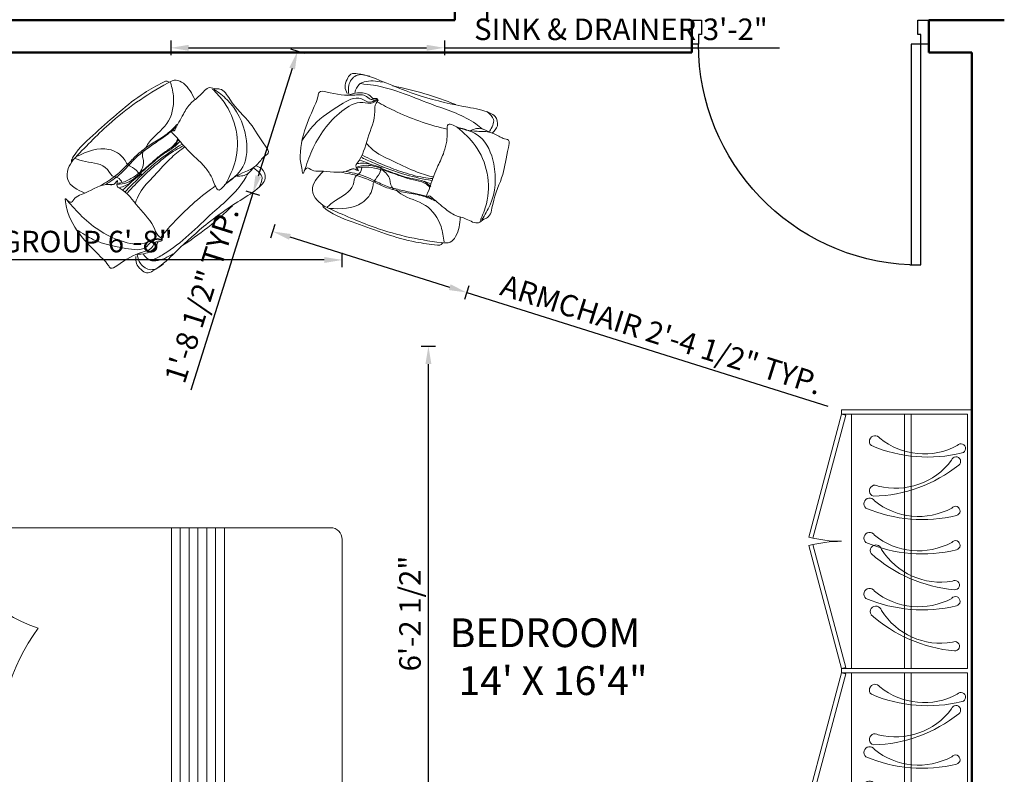
# Model space of a CAD drawing. Units: inches. Extents: x 1961 to 3038, y 800 to 1438.
# Tile 3 of 13: x 2666 to 2803, y 953 to 1058. Entities that reach past the tile are written whole.
import ezdxf

# ---------------------------------------------------------------- set-up
doc = ezdxf.new("R2010")
doc.units = ezdxf.units.IN
for name, color, linetype, lineweight in [('A-ANNO-DIMS', 2, 'Continuous', 18), ('A-AREA-IDEN', 7, 'Continuous', 25), ('A-DOOR', 3, 'Continuous', 25), ('A-FURN', 8, 'Continuous', 18), ('A-WALL', 7, 'Continuous', 50)]:
    doc.layers.add(name, color=color, linetype=linetype, lineweight=lineweight)
doc.styles.get("Standard").update_dxf_attribs({"font": 'arial.ttf'})
doc.dimstyles.new('ISO-25', dxfattribs={"dimtxt": 3, "dimasz": 2.5, "dimexe": 1, "dimexo": 1, "dimtad": 1, "dimdec": 4, "dimlunit": 4, "dimtxsty": 'Standard', "dimcen": 2.5, "dimadec": 0, "dimazin": 0, "dimtfac": 1, "dimtdec": 4, "dimtmove": 0, "dimatfit": 3, "dimfxl": 1, "dimfxlon": 1, "dimarcsym": 0})

# ---------------------------------------------------------------- blocks, each defined once
blk = doc.blocks.new('A$C41DA168A')
for p, q in [((151.4, 2380), (0, 1814.9)), ((19.3, 1809.8), (170.7, 2374.8)), ((151.4, 2380), (151.4, 2400)), ((151.4, 2400), (751.4, 2400)), ((731.4, 2380), (151.4, 2380)), ((170.7, 2374.8), (151.4, 2380)), ((196.6, 1210), (196.6, 2380)), ((441.4, 1210), (441.4, 2380)), ((471.4, 1210), (471.4, 2380)), ((731.4, 1210), (731.4, 2380)), ((751.4, 2400), (751.4, 0)), ((0, 1814.9), (19.3, 1809.8)), ((0, 1775.1), (19.3, 1780.2)), ((151.4, 1210), (0, 1775.1)), ((19.3, 1780.2), (170.7, 1215.2)), ((151.4, 1190), (0, 624.9)), ((19.3, 619.8), (170.7, 1184.8)), ((170.7, 1215.2), (151.4, 1210)), ((151.4, 1210), (731.4, 1210)), ((151.4, 1190), (151.4, 1210)), ((731.4, 1190), (151.4, 1190)), ((170.7, 1184.8), (151.4, 1190)), ((196.6, 20), (196.6, 1190)), ((441.4, 1190), (441.4, 20)), ((471.4, 1190), (471.4, 20)), ((731.4, 20), (731.4, 1190)), ((0, 624.9), (19.3, 619.8)), ((0, 585.1), (19.3, 590.2)), ((19.3, 590.2), (170.7, 25.2)), ((151.4, 20), (0, 585.1)), ((170.7, 25.2), (151.4, 20)), ((151.4, 0), (151.4, 20)), ((151.4, 20), (731.4, 20)), ((751.4, 0), (151.4, 0))]:
    blk.add_line(p, q)
for centre, radius, start, end in [((305.7, 2255.1), 26.3, 32.2752, 228.9651), ((530.9, 2518.7), 321.7, 230.8748, 298.3986), ((548.2, 2849.7), 667, 247.0836, 283.6394), ((700.5, 2222.3), 21.4, 283.2942, 141.1703), ((677.9, 2162.6), 21.4, 307.9992, 165.8752), ((277.3, 2668.9), 667, 271.7885, 308.3443), ((399.9, 2361), 321.7, 255.5797, 323.1036), ((305.5, 2027.4), 26.3, 56.9801, 253.67), ((280.2, 1967.6), 26.3, 32.2752, 228.9651), ((505.3, 2231.2), 321.7, 230.8748, 298.3986), ((675, 1934.8), 21.4, 283.2942, 141.1703), ((522.6, 2562.2), 667, 247.0836, 283.6394), ((151.4, 2380), 585, 255, 270), ((280.2, 1809.7), 26.3, 32.2752, 228.9651), ((505.3, 2073.2), 321.7, 230.8748, 298.3986), ((151.4, 1210), 585, 90, 105), ((522.6, 2404.2), 667, 247.0836, 283.6394), ((309.6, 1752), 26.3, 13.455, 210.1449), ((675, 1776.9), 21.4, 283.2942, 141.1703), ((730.9, 2236.5), 667, 228.2634, 264.8192), ((607.8, 1928.8), 321.7, 212.0546, 279.5785), ((672.7, 1593.6), 21.4, 264.474, 122.3501), ((280.2, 1552.2), 26.3, 32.2752, 228.9651), ((505.3, 1815.7), 321.7, 230.8748, 298.3986), ((675, 1519.4), 21.4, 283.2942, 141.1703), ((522.6, 2146.7), 667, 247.0836, 283.6394), ((309.6, 1470.8), 26.3, 13.455, 210.1449), ((730.9, 1955.3), 667, 228.2634, 264.8192), ((607.8, 1647.6), 321.7, 212.0546, 279.5785), ((672.7, 1312.3), 21.4, 264.474, 122.3501), ((305.7, 1111), 26.3, 32.2752, 228.9651), ((548.2, 1705.5), 667, 247.0836, 283.6394), ((530.9, 1374.6), 321.7, 230.8748, 298.3986), ((700.5, 1078.2), 21.4, 283.2942, 141.1703), ((277.3, 1524.8), 667, 271.7885, 308.3443), ((399.9, 1216.9), 321.7, 255.5797, 323.1036), ((677.9, 1018.5), 21.4, 307.9992, 165.8752), ((305.5, 883.3), 26.3, 56.9801, 253.67), ((280.2, 823.5), 26.3, 32.2752, 228.9651), ((505.3, 1087.1), 321.7, 230.8748, 298.3986), ((522.6, 1418), 667, 247.0836, 283.6394), ((675, 790.7), 21.4, 283.2942, 141.1703), ((280.2, 665.6), 26.3, 32.2752, 228.9651), ((505.3, 929.1), 321.7, 230.8748, 298.3986), ((522.6, 1260.1), 667, 247.0836, 283.6394), ((675, 632.8), 21.4, 283.2942, 141.1703), ((309.6, 607.9), 26.3, 13.455, 210.1449), ((730.9, 1092.4), 667, 228.2634, 264.8192), ((607.8, 784.7), 321.7, 212.0546, 279.5785), ((672.7, 449.5), 21.4, 264.474, 122.3501), ((280.2, 408.1), 26.3, 32.2752, 228.9651), ((505.3, 671.6), 321.7, 230.8748, 298.3986), ((522.6, 1002.6), 667, 247.0836, 283.6394), ((675, 375.3), 21.4, 283.2942, 141.1703), ((309.6, 326.7), 26.3, 13.455, 210.1449), ((607.8, 503.5), 321.7, 212.0546, 279.5785), ((730.9, 811.2), 667, 228.2634, 264.8192), ((672.7, 168.2), 21.4, 264.474, 122.3501)]:
    blk.add_arc(centre, radius, start, end)
blk = doc.blocks.new('A$C11850ECD')
for p, q in [((0, 1.95), (0, 0.04)), ((0, 1.95), (1.2, 1.95)), ((1.2, 1.95), (1.2, 0.04)), ((1.2318, 1.952), (1.8168, 1.952)), ((1.2318, 1.367), (1.2318, 1.952)), ((1.5243, 1.952), (1.5243, 1.7225)), ((1.8168, 1.952), (1.8168, 1.367)), ((0, 1.91), (1.2, 1.91)), ((0, 1.9), (1.2, 1.9)), ((1.4613, 1.6586), (1.2318, 1.6586)), ((1.8168, 1.6595), (1.5873, 1.6595)), ((1.5243, 1.5965), (1.5243, 1.367)), ((1.8168, 1.367), (1.2318, 1.367)), ((0, 0.58), (1.2, 0.58)), ((0, 0.55), (1.2, 0.55)), ((0, 0.52), (1.2, 0.52)), ((0, 0.49), (1.2, 0.49)), ((0, 0.46), (1.2, 0.46)), ((0, 0.43), (1.2, 0.43)), ((0, 0.4), (1.2, 0.4)), ((1.16, 0), (0.04, 0))]:
    blk.add_line(p, q)
for radius in [0.27, 0.09]:
    blk.add_circle((1.5243, 1.6595), radius)
for centre, radius, start, end in [((-0.2053, 1.694), 0.5605, 346.15, 13.85), ((0.5998, 5.1077), 3.2899, 265.4501, 274.5499), ((0.3425, 1.5416), 0.3789, 4.7708, 46.8165), ((0.3425, 1.5416), 0.4089, 4.1373, 42.5614), ((0.3425, 1.5416), 0.4389, 3.5318, 39.1874), ((0.3425, 1.5416), 0.4689, 2.9489, 36.4321), ((1.3429, 1.694), 0.5004, 164.4468, 195.5532), ((0.5998, -0.4629), 2.0395, 82.6483, 97.3517), ((0.8389, 0.3894), 1.0202, 69.2731, 145.3133), ((1.3044, 0.8859), 0.4695, 102.8515, 161.769), ((0.4655, 0.5058), 0.6574, 53.2823, 135.0802), ((0.04, 0.04), 0.04, 180, 270), ((1.16, 0.04), 0.04, 270, 0)]:
    blk.add_arc(centre, radius, start, end)
blk = doc.blocks.new('A$C4F7F6E58')
at = {"ltscale": 0.8}
blk.add_arc((588.7, 1807.5), 1799.5, 263.3519, 274.6778, dxfattribs=at)
for points, knots in [([(212.3, 745.6), (213, 747.1), (218.5, 755.7), (289.3, 782.2), (464.8, 786.6), (683, 801.1), (833.5, 773.4), (885.9, 762.1), (890.8, 751.2), (892, 745.8)], [17.99656, 17.99656, 17.99656, 17.99656, 24.654541, 59.355785, 289.542515, 728.551681, 882.30278, 904.288941, 924.788376, 924.788376, 924.788376, 924.788376]), ([(227.7, 750.3), (210.2, 745.1), (173.8, 734.3), (112.7, 672.2), (142.7, 611.7), (162.7, 571.5)], [0, 0, 0, 0, 71.10826, 148.314414, 301.164142, 301.164142, 301.164142, 301.164142]), ([(227.7, 750.3), (317.7, 761.3), (538, 788.2), (765.4, 771.9), (932.7, 737.6), (960.4, 670.7), (949, 620.8), (940.8, 585)], [0, 0, 0, 0, 350.70006, 858.205579, 917.075962, 972.848208, 1113.682742, 1113.682742, 1113.682742, 1113.682742]), ([(238.5, 752.4), (248.9, 735.1), (280.7, 682.5), (353.2, 623), (328.1, 546.3), (358.7, 520.1), (356, 500.2), (354.3, 487.1)], [0, 0, 0, 0, 79.489254, 242.739997, 314.65082, 339.438853, 386.590051, 386.590051, 386.590051, 386.590051]), ([(251.9, 753.3), (314, 736.9), (407.7, 709), (450.5, 599.8), (436.6, 550.7), (446.8, 516.8), (458.3, 488.6), (454.8, 465.3), (454.1, 460.2)], [14.22546, 14.22546, 14.22546, 14.22546, 248.732969, 375.734785, 418.155281, 441.003934, 511.971111, 531.951261, 531.951261, 531.951261, 531.951261]), ([(897.7, 739.5), (885.8, 714.1), (853.7, 645.7), (745.6, 561.4), (631.8, 577.3), (575.9, 554.3), (565.2, 549.9)], [0, 0, 0, 0, 109.257629, 294.294606, 484.078985, 528.781997, 528.781997, 528.781997, 528.781997]), ([(85.7, 579.8), (108.8, 591.2), (183.8, 558.4), (269.7, 555.1), (310.5, 503.2), (358.6, 519.6), (314.2, 495.4), (342.8, 432.7), (331.4, 330.5), (346.7, 210.6), (316.5, 146.3), (334, 110.2), (306.1, 110.8), (292.3, 132.5), (251.9, 105.6), (169.8, 145.3), (100.6, 155.5), (8.5, 162.1), (15.1, 200), (9.7, 271), (-8.6, 395.1), (11.8, 535.4), (46.6, 590.2), (64.4, 626.1), (63, 591.9), (73.2, 578.8), (82.8, 578.4), (85.7, 579.8)], [0, 0, 0, 0, 100.597406, 281.319891, 315.054718, 349.509689, 389.200281, 408.162693, 598.959573, 792.637569, 852.601939, 880.830983, 902.666946, 929.495226, 968.022274, 1050.611483, 1254.96923, 1301.260424, 1329.316584, 1382.311494, 1591.546287, 1820.820862, 1871.094845, 1893.578982, 1925.370652, 1945.336599, 1957.814292, 1957.814292, 1957.814292, 1957.814292]), ([(64.1, 601.9), (65, 562.5), (67.9, 434.1), (120.6, 270.6), (224.7, 149.7), (303.4, 150.5), (317.5, 124.2), (323, 114)], [0, 0, 0, 0, 153.199383, 498.931474, 658.942203, 726.134726, 768.614124, 768.614124, 768.614124, 768.614124]), ([(752, 526.5), (782.1, 539.3), (834.3, 561.4), (909.8, 589.7), (975.3, 580.2), (1040.8, 601.3), (1061.5, 560.1), (1098.2, 533.5), (1075.6, 429.8), (1100.1, 301), (1076.9, 198.1), (1073.4, 103.2), (1039.5, 112.8), (1006.2, 107.3), (957.4, 94.2), (871.3, 124.9), (803.4, 133.9), (712.9, 116.6), (740.5, 179.9), (750.1, 225.2), (754, 285.2), (740.4, 365.6), (734.8, 446.5), (737.4, 494.3), (727.2, 554.4), (746.7, 524.2), (752, 526.5)], [0, 0, 0, 0, 127.427681, 224.276404, 302.261986, 392.779016, 437.096694, 463.557063, 563.507143, 784.838909, 976.246821, 1028.506194, 1069.058754, 1082.809516, 1162.638681, 1258.731906, 1422.314775, 1462.867277, 1544.873185, 1583.434163, 1661.617215, 1768.019408, 1911.553131, 1945.84397, 1998.930645, 2021.420543, 2021.420543, 2021.420543, 2021.420543]), ([(253, 547.9), (286.3, 543.8), (348.1, 536.3), (432.8, 543.6), (496.9, 552.8), (560.5, 553.7), (630.5, 546.9), (709.3, 534), (761.1, 540.1), (783.5, 542.8)], [0, 0, 0, 0, 130.481225, 241.871234, 329.653071, 382.635961, 489.129551, 603.809277, 691.391283, 691.391283, 691.391283, 691.391283]), ([(279.6, 536), (309.9, 532.6), (359.7, 527), (435.7, 535.5), (505.5, 548.5), (584.2, 543.4), (656.3, 537.7), (718.8, 532.6), (754.3, 534.8), (769.2, 535.7)], [0, 0, 0, 0, 118.476382, 194.076844, 297.117853, 393.933927, 499.659542, 579.515716, 637.850776, 637.850776, 637.850776, 637.850776]), ([(551.9, 549.7), (549.4, 547.7), (542.3, 542.2), (527, 531), (516.3, 490.8), (483.3, 477.5), (459.7, 467.9)], [0, 0, 0, 0, 12.396318, 35.253043, 71.848794, 163.317226, 163.317226, 163.317226, 163.317226]), ([(1056.3, 563.2), (1063.7, 533.8), (1089.5, 431.8), (1051.6, 268.9), (926.4, 121.9), (821.2, 125.9), (773.1, 127.7)], [0, 0, 0, 0, 117.484834, 407.414781, 620.246611, 799.395046, 799.395046, 799.395046, 799.395046]), ([(1050, 569.3), (1052.8, 537.7), (1065, 399.7), (962.6, 208.3), (822.2, 146.8), (780.2, 128.4)], [0, 0, 0, 0, 123.587716, 539.784626, 717.53011, 717.53011, 717.53011, 717.53011]), ([(325.5, 498.4), (341, 486.6), (382.1, 460.9), (458.6, 463.7), (543.1, 467.4), (620.7, 469.4), (690.3, 455.1), (724.9, 469.5), (738.9, 475.3)], [49.606189, 49.606189, 49.606189, 49.606189, 124.052713, 239.571345, 333.3214, 456.942517, 542.38691, 600.329448, 600.329448, 600.329448, 600.329448]), ([(328.4, 501.8), (338.5, 496), (366.7, 480), (433, 469.7), (510.6, 467.3), (589.8, 472.9), (650.9, 468.8), (701.4, 464), (726.3, 476.5), (736.2, 481.5)], [0, 0, 0, 0, 45.174964, 125.558829, 256.610972, 349.076861, 433.189907, 497.197145, 539.983253, 539.983253, 539.983253, 539.983253]), ([(2.6, 449.8), (13.4, 414.5), (41.8, 321.3), (126.7, 222.3), (214.2, 117.7), (295.4, 153.1), (311.3, 117.2), (325.2, 118), (331.2, 118.3)], [0, 0, 0, 0, 141.86292, 373.630524, 526.427539, 601.735045, 630.296438, 651.966247, 651.966247, 651.966247, 651.966247]), ([(323.9, 476.4), (335.1, 471.9), (362.5, 460.9), (411, 458.3), (446.9, 458.3), (465.4, 458.3)], [0, 0, 0, 0, 46.593931, 114.59593, 186.8347, 186.8347, 186.8347, 186.8347]), ([(330.8, 455.3), (347.2, 455.7), (369, 456.2), (390.6, 458.7), (395.9, 459.3)], [0, 0, 0, 0, 63.690529, 84.680578, 84.680578, 84.680578, 84.680578]), ([(338.1, 439.1), (365.6, 442.5), (450.6, 453.1), (583.9, 460.6), (688.5, 449), (735.4, 443.9)], [0, 0, 0, 0, 108.049196, 333.891802, 517.629591, 517.629591, 517.629591, 517.629591]), ([(339.5, 358.4), (356.3, 367.8), (409.4, 397.6), (517.2, 404.8), (632.4, 427.1), (708.8, 424.4), (739.9, 423.2)], [0, 0, 0, 0, 74.526832, 235.368216, 411.08678, 532.069418, 532.069418, 532.069418, 532.069418]), ([(340.4, 426.7), (378.9, 432.1), (452.3, 442.3), (568.3, 448.5), (663.3, 447.1), (721.2, 435), (737.7, 431.5)], [0, 0, 0, 0, 151.37946, 288.564606, 452.874576, 518.766039, 518.766039, 518.766039, 518.766039]), ([(326.5, 126.4), (359.8, 134.8), (489.4, 155.9), (624.9, 163.3), (724.8, 154.9), (728.6, 154.6)], [89.052228, 89.052228, 89.052228, 89.052228, 222.96578, 599.021538, 613.61065, 613.61065, 613.61065, 613.61065]), ([(158.9, 133), (150.2, 123.2), (131.9, 102.7), (133.9, 63.3), (141.9, 22.3), (217.8, 4.9), (345.6, 16.6), (555.4, 32.4), (757.1, 15.8), (894.9, -4.6), (965.2, 8.9), (992.9, 55.8), (976.8, 87.4), (969, 102.7)], [0, 0, 0, 0, 48.943013, 103.025949, 148.534553, 195.328972, 375.361256, 667.155028, 1003.182997, 1165.538814, 1206.58239, 1274.47318, 1338.225006, 1338.225006, 1338.225006, 1338.225006]), ([(169.5, 134.2), (162.3, 119.5), (145.6, 84.9), (169.5, 11.7), (220.8, 8.8), (248.3, 7.3)], [0, 0, 0, 0, 62.883797, 147.829924, 245.663948, 245.663948, 245.663948, 245.663948]), ([(165.8, 141.2), (180, 130.6), (212.9, 106.1), (268, 97.7), (294.2, 114.6), (300.7, 118.8)], [0, 0, 0, 0, 69.56601, 160.233414, 189.860891, 189.860891, 189.860891, 189.860891]), ([(196.7, 116), (197, 98.2), (197.4, 70), (245.3, 28.7), (288.9, 22), (322.6, 16.8)], [0, 0, 0, 0, 65.355661, 103.354857, 233.394712, 233.394712, 233.394712, 233.394712]), ([(855.5, 122.2), (863.4, 115.5), (886.8, 95.7), (925.1, 92.8), (947, 101), (950.1, 102.2)], [0, 0, 0, 0, 40.128951, 118.809172, 131.501248, 131.501248, 131.501248, 131.501248]), ([(912.5, 96.7), (898.4, 91.1), (808.6, 55.2), (592.1, 57.5), (371.7, 28.4), (235.4, 55.8), (212.6, 60.4)], [0, 0, 0, 0, 58.661068, 375.93507, 825.814021, 916.361162, 916.361162, 916.361162, 916.361162]), ([(952.5, 98), (958.3, 72.4), (968.9, 25.7), (925.9, 8), (906.6, 0)], [0, 0, 0, 0, 88.639768, 160.999132, 160.999132, 160.999132, 160.999132])]:
    blk.add_open_spline(points, degree=3, knots=knots, dxfattribs=at)
for points in [[(295.1, 523.4), (300.3, 519), (305.5, 514.5), (310.7, 510.2)], [(736.1, 462.3), (723.2, 461.1), (710.3, 459.9), (697.4, 458.7)]]:
    blk.add_open_spline(points, degree=3, dxfattribs=at)
blk = doc.blocks.new('DOOR-SWING-33IN')
for p, q in [((30.36, 34.07), (31.87, 34.07)), ((30.53, 3.34), (30.53, 34.07)), ((31.87, 34.07), (31.87, 3.34)), ((33, 3.34), (30.53, 3.34)), ((31.87, 3.34), (31.87, 2)), ((31.87, 2), (31.46, 2)), ((31.46, 2), (31.46, 0)), ((31.46, 0), (33, 0))]:
    blk.add_line(p, q)
blk.add_lwpolyline([(0, 0), (1.34, 0), (1.34, 2), (0.93, 2), (0.93, 3.34), (0, 3.34)])
blk.add_arc((31.69, 3.34), 30.76, 92.4896, 180)
blk = doc.blocks.new('*D39')
at = {"layer": 'A-ANNO-DIMS', "color": 0, "lineweight": -2, "transparency": 16777216}
for p, q in [((2701.72, 1029.95), (2701.12, 1028.04)), ((2703.81, 1028.24), (2726.04, 1021.24)), ((2728.73, 1021.44), (2728.13, 1019.53)), ((2728.43, 1020.49), (2778.71, 1004.65))]:
    blk.add_line(p, q, dxfattribs=at)
at = {"layer": 'A-ANNO-DIMS', "color": 0, "transparency": 16777216}
for points in [[(2703.93, 1028.64), (2703.68, 1027.85), (2701.42, 1028.99)], [(2726.17, 1021.64), (2725.92, 1020.84), (2728.43, 1020.49)]]:
    blk.add_solid(points, dxfattribs=at)
at = {"layer": 'Defpoints', "color": 0, "transparency": 16777216}
for p in [(2702.7, 1033.05), (2729.7, 1024.54), (2728.43, 1020.49)]:
    blk.add_point(p, dxfattribs=at)
at = {"layer": 'A-ANNO-DIMS', "color": 0, "transparency": 16777216, "insert": (2755.42, 1014.27), "char_height": 3, "attachment_point": 5, "rotation": 342.5185}
blk.add_mtext('ARMCHAIR 2\'-4 1/2" TYP.', dxfattribs=at)
blk = doc.blocks.new('*D40')
at = {"layer": 'A-ANNO-DIMS', "color": 0, "lineweight": -2, "transparency": 16777216}
for p, q in [((2705.82, 1053.76), (2703.91, 1054.36)), ((2704.11, 1051.68), (2699.4, 1036.71)), ((2698.65, 1034.32), (2690.01, 1006.9)), ((2699.6, 1034.02), (2697.69, 1034.62))]:
    blk.add_line(p, q, dxfattribs=at)
at = {"layer": 'A-ANNO-DIMS', "color": 0, "transparency": 16777216}
for points in [[(2703.71, 1051.8), (2704.51, 1051.55), (2704.86, 1054.06)], [(2699, 1036.83), (2699.79, 1036.58), (2698.65, 1034.32)]]:
    blk.add_solid(points, dxfattribs=at)
at = {"layer": 'Defpoints', "color": 0, "transparency": 16777216}
for p in [(2708.91, 1052.78), (2698.65, 1034.32), (2702.7, 1033.05)]:
    blk.add_point(p, dxfattribs=at)
at = {"layer": 'A-ANNO-DIMS', "color": 0, "transparency": 16777216, "insert": (2691.88, 1020.07), "char_height": 3, "attachment_point": 5, "rotation": 72.5185}
blk.add_mtext('1\'-8 1/2" TYP.', dxfattribs=at)
blk = doc.blocks.new('*D57')
at = {"layer": 'A-ANNO-DIMS', "color": 0, "lineweight": -2, "transparency": 16777216}
for p, q in [((2631.09, 1024.03), (2631.09, 1026.03)), ((2711.09, 1024.03), (2711.09, 1026.03)), ((2708.59, 1025.03), (2633.59, 1025.03))]:
    blk.add_line(p, q, dxfattribs=at)
at = {"layer": 'A-ANNO-DIMS', "color": 0, "transparency": 16777216}
for points in [[(2633.59, 1025.44), (2633.59, 1024.61), (2631.09, 1025.03)], [(2708.59, 1025.44), (2708.59, 1024.61), (2711.09, 1025.03)]]:
    blk.add_solid(points, dxfattribs=at)
at = {"layer": 'Defpoints', "color": 0, "transparency": 16777216}
for p in [(2631.09, 1025.03), (2631.09, 1013.03), (2711.09, 1013.03)]:
    blk.add_point(p, dxfattribs=at)
at = {"layer": 'A-ANNO-DIMS', "color": 0, "transparency": 16777216, "insert": (2671.09, 1027.2), "char_height": 3, "attachment_point": 5}
blk.add_mtext('BED GROUP 6\'-8"', dxfattribs=at)
blk = doc.blocks.new('*D58')
at = {"layer": 'A-ANNO-DIMS', "color": 0, "lineweight": -2, "transparency": 16777216}
for p, q in [((2722.09, 1013.03), (2724.09, 1013.03)), ((2723.09, 941.07), (2723.09, 1010.53)), ((2722.09, 938.57), (2724.09, 938.57))]:
    blk.add_line(p, q, dxfattribs=at)
at = {"layer": 'A-ANNO-DIMS', "color": 0, "transparency": 16777216}
for points in [[(2722.67, 1010.53), (2723.5, 1010.53), (2723.09, 1013.03)], [(2722.67, 941.07), (2723.5, 941.07), (2723.09, 938.57)]]:
    blk.add_solid(points, dxfattribs=at)
at = {"layer": 'Defpoints', "color": 0, "transparency": 16777216}
for p in [(2711.09, 1013.03), (2723.09, 1013.03), (2711.09, 938.57)]:
    blk.add_point(p, dxfattribs=at)
at = {"layer": 'A-ANNO-DIMS', "color": 0, "transparency": 16777216, "insert": (2720.91, 975.8), "char_height": 3, "attachment_point": 5, "rotation": 90}
blk.add_mtext('6\'-2 1/2"', dxfattribs=at)
blk = doc.blocks.new('*D69')
at = {"layer": 'A-ANNO-DIMS', "color": 0, "lineweight": -2, "transparency": 16777216}
for p, q in [((2687.2, 1055.56), (2687.2, 1053.56)), ((2689.7, 1054.56), (2722.82, 1054.56)), ((2725.32, 1055.56), (2725.32, 1053.56)), ((2725.32, 1054.56), (2771.96, 1054.56))]:
    blk.add_line(p, q, dxfattribs=at)
at = {"layer": 'A-ANNO-DIMS', "color": 0, "transparency": 16777216}
for points in [[(2689.7, 1054.98), (2689.7, 1054.15), (2687.2, 1054.56)], [(2722.82, 1054.98), (2722.82, 1054.15), (2725.32, 1054.56)]]:
    blk.add_solid(points, dxfattribs=at)
at = {"layer": 'Defpoints', "color": 0, "transparency": 16777216}
for p in [(2687.2, 1060.28), (2725.32, 1060.28), (2725.32, 1054.56)]:
    blk.add_point(p, dxfattribs=at)
at = {"layer": 'A-ANNO-DIMS', "color": 0, "transparency": 16777216, "insert": (2749.89, 1056.75), "char_height": 3, "attachment_point": 5}
blk.add_mtext('SINK & DRAINER 3\'-2"', dxfattribs=at)

msp = doc.modelspace()

# ---------------------------------------------------------------- linework, layer by layer
at = {"layer": 'A-WALL'}
for p, q in [((2726.76803, 1124.41975), (2726.76803, 1058.41975)), ((2731.26803, 1124.41975), (2731.26803, 1058.41975)), ((2726.76803, 1058.41975), (2630.76803, 1058.41975)), ((2759.76803, 1058.41975), (2759.76803, 1053.91975)), ((2803.26803, 1058.41975), (2792.76803, 1058.41975)), ((2792.76803, 1058.41975), (2792.76803, 1053.91975)), ((2759.76803, 1053.91975), (2630.76803, 1053.91975)), ((2798.76803, 1053.91975), (2792.76803, 1053.91975)), ((2798.76803, 1053.91975), (2798.76803, 858.91975))]:
    msp.add_line(p, q, dxfattribs=at)

# ---------------------------------------------------------------- block references
at = {"layer": 'A-DOOR', "extrusion": (0, 0, -1), "zscale": -1, "rotation": 180}
msp.add_blockref('DOOR-SWING-33IN', (-2759.768, 1058.41951), dxfattribs=at)
at = {"layer": 'A-FURN'}
for name, p, xscale, yscale, zscale, rotation in [('A$C4F7F6E58', (2681.36471, 1020.26477), 0.0258216611436376, 0.0258216611436376, 0.0258216611436376, 39.33090782219615), ('A$C4F7F6E58', (2708.89155, 1052.70849), -0.0258216611436376, 0.0258216611436376, 0.0258216611436376, 162.5185450702014), ('A$C11850ECD', (2711.08548, 938.57032), 40.98381615062051, 40.98381615062051, 40.98381615062051, 90)]:
    msp.add_blockref(name, p, dxfattribs=dict(at, xscale=xscale, yscale=yscale, zscale=zscale, rotation=rotation))
at = {"layer": 'A-FURN', "xscale": 0.0302586277246643, "yscale": 0.0302586277246643, "zscale": 0.0302586277246643}
msp.add_blockref('A$C41DA168A', (2776.03142, 931.54046), dxfattribs=at)

# ---------------------------------------------------------------- texts
at = {"layer": 'A-AREA-IDEN', "insert": (2726.04117, 975.12586), "char_height": 4, "attachment_point": 1}
msp.add_mtext_dynamic_manual_height_columns('{\\fTimes New Roman|b1|i0|c0|p18;BEDROOM\\P 14\' X 16\'4"}', width=33.1080891, gutter_width=12.5, heights=[0], dxfattribs=at)

# ---------------------------------------------------------------- dimensions: what is measured, and where the dimension line sits
at = {"layer": 'A-ANNO-DIMS'}
dim = msp.add_linear_dim(base=(2725.32185, 1054.56259), p1=(2687.20225, 1060.28053), p2=(2725.32185, 1060.28053), text='SINK & DRAINER <>', dimstyle='ISO-25', override={"dimdec": 1, "dimlfac": 1, "dimrnd": 0, "dimzin": 1, "dimdsep": 46, "dimlunit": 4, "dimfrac": 2}, dxfattribs=at)
dim.commit()
dim.dimension.update_dxf_attribs({"geometry": '*D69', "text_midpoint": (2749.89296, 1056.74796)})
for base, p1, p2, angle, text, picture, middle in [((2698.64539, 1034.32104), (2708.91298, 1052.7837), (2702.69648, 1033.04518), 252.5185451, '<> TYP.', '*D40', (2691.87686, 1020.07401)), ((2631.08548, 1025.02777), (2711.08548, 1013.02777), (2631.08548, 1013.02777), 180, 'BED GROUP <>', '*D57', (2671.08548, 1027.20495)), ((2728.42782, 1020.48837), (2702.69648, 1033.04518), (2729.70368, 1024.53945), 342.5185451, 'ARMCHAIR <> TYP.', '*D39', (2755.41536, 1014.27037))]:
    dim = msp.add_linear_dim(base=base, p1=p1, p2=p2, angle=angle, text=text, dimstyle='ISO-25', override={"dimdec": 1, "dimlfac": 1, "dimrnd": 0, "dimzin": 1, "dimdsep": 46, "dimlunit": 4, "dimfrac": 2}, dxfattribs=at)
    dim.commit()
    dim.dimension.update_dxf_attribs({"geometry": picture, "text_midpoint": middle})
dim = msp.add_linear_dim(base=(2723.08548, 1013.02777), p1=(2711.08548, 938.57031), p2=(2711.08548, 1013.02777), angle=90, dimstyle='ISO-25', override={"dimdec": 1, "dimlfac": 1, "dimrnd": 0, "dimzin": 1, "dimdsep": 46, "dimlunit": 4, "dimfrac": 2}, dxfattribs=at)
dim.commit()
dim.dimension.update_dxf_attribs({"geometry": '*D58', "text_midpoint": (2720.90932, 975.79904)})

doc.saveas('drawing.dxf')
